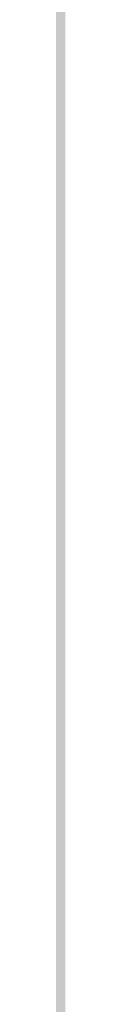
# Model space of a CAD drawing. Units: inches. Extents: x 2083 to 3317, y 1141 to 2115.
# Tile 219 of 256: x 3126.956 to 3126.958, y 1265.165 to 1267.234. Entities that reach past the tile are written whole.
import ezdxf

# ---------------------------------------------------------------- set-up
doc = ezdxf.new("R2010")
doc.units = ezdxf.units.IN
doc.layers.add('A-ANNO-DIMS', color=2, linetype='Continuous', lineweight=18)
doc.layers.add('A-WALL-PATT', color=251, linetype='Continuous', lineweight=13, true_color=0x636466)
doc.styles.get("Standard").update_dxf_attribs({"font": 'arial.ttf'})
doc.dimstyles.new('ISO-25', dxfattribs={"dimtxt": 12, "dimasz": 12, "dimexe": 1.25, "dimexo": 0.625, "dimtad": 1, "dimlunit": 3, "dimtxsty": 'Standard', "dimcen": 2.5, "dimadec": 0, "dimazin": 0, "dimtfac": 1, "dimtmove": 0, "dimatfit": 3, "dimfxl": 1, "dimarcsym": 0})

# ---------------------------------------------------------------- blocks, each defined once
blk = doc.blocks.new('*D26')
at = {"layer": 'A-ANNO-DIMS', "color": 0, "lineweight": -2, "transparency": 16777216}
for p, q in [((3088.9858, 1274.9151), (3088.9858, 1270.952)), ((3111.24, 1274.9151), (3111.24, 1270.952)), ((3076.9858, 1272.202), (2840.2624, 1272.202)), ((3111.24, 1272.202), (3088.9858, 1272.202)), ((3123.24, 1272.202), (3135.24, 1272.202))]:
    blk.add_line(p, q, dxfattribs=at)
at = {"layer": 'A-ANNO-DIMS', "color": 0, "transparency": 16777216}
for points in [[(3076.9858, 1274.202), (3076.9858, 1270.202), (3088.9858, 1272.202)], [(3123.24, 1274.202), (3123.24, 1270.202), (3111.24, 1272.202)]]:
    blk.add_solid(points, dxfattribs=at)
at = {"layer": 'Defpoints', "color": 0, "transparency": 16777216}
for p in [(3088.9858, 1275.5401), (3111.24, 1275.5401), (3088.9858, 1272.202)]:
    blk.add_point(p, dxfattribs=at)
at = {"layer": 'A-ANNO-DIMS', "color": 0, "transparency": 16777216, "insert": (2952.6241, 1279.0316), "char_height": 12, "attachment_point": 5}
blk.add_mtext('NIGHTSTAND 1\'-10 1/2" TYP.', dxfattribs=at)
blk = doc.blocks.new('*D27')
at = {"layer": 'A-ANNO-DIMS', "color": 0, "lineweight": -2, "transparency": 16777216}
for p, q in [((3114.5782, 1309.7943), (3114.5782, 1321.7943)), ((3111.865, 1297.7943), (3115.8282, 1297.7943)), ((3114.5782, 1297.7943), (3114.5782, 1275.5401)), ((3111.865, 1275.5401), (3115.8282, 1275.5401)), ((3114.5782, 1263.5401), (3114.5782, 1140.9886))]:
    blk.add_line(p, q, dxfattribs=at)
at = {"layer": 'A-ANNO-DIMS', "color": 0, "transparency": 16777216}
for points in [[(3112.5782, 1309.7943), (3116.5782, 1309.7943), (3114.5782, 1297.7943)], [(3112.5782, 1263.5401), (3116.5782, 1263.5401), (3114.5782, 1275.5401)]]:
    blk.add_solid(points, dxfattribs=at)
at = {"layer": 'Defpoints', "color": 0, "transparency": 16777216}
for p in [(3111.24, 1297.7943), (3111.24, 1275.5401), (3114.5782, 1275.5401)]:
    blk.add_point(p, dxfattribs=at)
at = {"layer": 'A-ANNO-DIMS', "color": 0, "transparency": 16777216, "insert": (3107.7485, 1196.2643), "char_height": 12, "attachment_point": 5, "rotation": 90}
blk.add_mtext('1\'-10 1/2" TYP.', dxfattribs=at)

msp = doc.modelspace()

# ---------------------------------------------------------------- hatches: boundary and pattern name
at = {"layer": 'A-WALL-PATT'}
h = msp.add_hatch(color=256, dxfattribs=at)
h.dxf.hatch_style = 1
h.paths.add_polyline_path([(3126.9598, 2020.7614), (2748.9598, 2020.7614), (2604.9598, 2020.7614), (2226.9598, 2020.7614), (2226.9598, 1702.7614), (2466.9598, 1702.7614), (2466.9598, 1582.7614), (2418.9598, 1582.7614), (2418.9598, 1477.7614), (2226.9598, 1477.7614), (2226.9598, 1263.2614), (2544.9598, 1263.2614), (2544.9598, 1411.7614), (2604.9598, 1411.7614), (2685.9598, 1411.7614), (2685.9598, 1420.7614), (2604.9598, 1420.7614), (2604.9598, 1573.7614), (2604.9598, 1702.7614), (2604.9598, 2011.7614), (2748.9598, 2011.7614), (2748.9598, 1702.7614), (2862.9598, 1702.7614), (2862.9598, 1621.7614), (2871.9598, 1621.7614), (2871.9598, 1702.7614), (2883.9598, 1702.7614), (2883.9598, 1706.9395, -0.026459), (2883.9598, 1711.7614), (2757.9598, 1711.7614), (2757.9598, 1807.7614), (2787.9598, 1807.7614), (2787.9598, 1812.2614), (2757.9598, 1812.2614), (2757.9598, 2011.7614), (2877.9598, 2011.7614), (2877.9598, 1812.2614), (2847.9598, 1812.2614), (2847.9598, 1807.7614), (2889.8357, 1807.7614), (2889.8357, 1812.2614), (2882.4598, 1812.2614), (2882.4598, 2011.7614), (3117.9598, 2011.7614), (3117.9598, 1812.2614), (2937.8357, 1812.2614), (2937.8357, 1807.7614), (2995.7098, 1807.7614), (2995.7098, 1796.1177), (3000.2098, 1796.1177), (3000.2098, 1807.7614), (3117.9598, 1807.7614), (3117.9598, 1711.7614), (3000.2098, 1711.7614), (3000.2098, 1760.1177), (2998.5727, 1760.1177, -0.020711), (2995.7098, 1760.1177), (2995.7098, 1711.7614), (2931.9598, 1711.7614), (2931.9598, 1702.7614), (3126.9598, 1702.7614)])
h.paths.add_polyline_path([(2471.4598, 2011.7614), (2471.4598, 1810.0114), (2462.7169, 1810.0114), (2462.7169, 1805.5114), (2505.9598, 1805.5114), (2505.9598, 1810.0114), (2475.9598, 1810.0114), (2475.9598, 2011.7614), (2595.9598, 2011.7614), (2595.9598, 1810.0114), (2565.9598, 1810.0114), (2565.9598, 1805.5114), (2595.9598, 1805.5114), (2595.9598, 1711.7614), (2235.9598, 1711.7614), (2235.9598, 1805.5114), (2353.7098, 1805.5114), (2353.7098, 1796.0542), (2358.2098, 1796.0542), (2358.2098, 1805.5114), (2414.7169, 1805.5114), (2414.7169, 1810.0114), (2235.9598, 1810.0114), (2235.9598, 2011.7614)], flags=16)
h.paths.add_polyline_path([(2270.2047, 1994.61), (2270.2047, 1970.61), (2246.2047, 1970.61), (2246.2047, 1994.61)], flags=0)
edge = h.paths.add_edge_path(flags=0)
edge.add_ellipse((2332.0274, 1899.7982), major_axis=(-3.043, 3.043), ratio=0.168252, start_angle=-161.3322, end_angle=-156.3071, ccw=False)
edge.add_ellipse((2333.082, 1898.7435), major_axis=(-1.0546, 1.0546), ratio=0.453532, start_angle=-123.371, end_angle=-94.1591)
edge = h.paths.add_edge_path(flags=0)
edge.add_ellipse((2332.0274, 1968.8763), major_axis=(3.043, 3.043), ratio=0.168252, start_angle=18.6678, end_angle=23.6929)
edge.add_spline(control_points=[(2332.9256, 1970.6911), (2332.2268, 1970.3361), (2330.8937, 1969.6589), (2328.4131, 1970.9321), (2327.2039, 1967.7487), (2324.7096, 1969.9556), (2322.5328, 1967.0124), (2320.0128, 1971.2958), (2317.6803, 1968.1578), (2316.0405, 1967.102), (2315.4269, 1966.8096)], knot_values=[0, 0, 0, 0, 2.267059, 4.324559, 6.685584, 8.878641, 11.121502, 14.300359, 17.755284, 19.732645, 19.732645, 19.732645, 19.732645], degree=3, periodic=0)
edge.add_ellipse((2332.0274, 1968.8763), major_axis=(3.043, 3.043), ratio=0.168252, start_angle=18.6678, end_angle=23.6929, ccw=False)
edge.add_ellipse((2333.082, 1969.9309), major_axis=(1.0546, 1.0546), ratio=0.453532, start_angle=56.629, end_angle=85.8409, ccw=False)
edge = h.paths.add_edge_path(flags=0)
edge.add_spline(control_points=[(2296.4283, 1967.9879), (2293.6278, 1965.3363), (2287.7036, 1959.7271), (2299.7439, 1949.9957), (2294.5326, 1935.6685), (2290.5732, 1920.6035), (2293.3941, 1909.9737), (2296.1854, 1904.9665)], knot_values=[0.099185, 0.099185, 0.099185, 0.099185, 0.345301, 0.619822, 0.982653, 1.386093, 1.810555, 1.810555, 1.810555, 1.810555], degree=3, periodic=0)
edge.add_spline(control_points=[(2296.1854, 1904.9665), (2297.3836, 1902.6193), (2298.001, 1901.9493), (2298.553, 1901.4682)], knot_values=[0.006246, 0.006246, 0.006246, 0.006246, 0.055476, 0.055476, 0.055476, 0.055476], degree=3, periodic=0)
edge.add_spline(control_points=[(2298.553, 1901.4682), (2297.2586, 1900.9232), (2295.2253, 1900.2321), (2293.0602, 1900.6142), (2292.1014, 1900.7884), (2292.0896, 1900.7906)], knot_values=[0.312835, 0.312835, 0.312835, 0.312835, 0.40178, 0.474987, 0.475903, 0.475903, 0.475903, 0.475903], degree=3, periodic=0)
edge.add_arc((2292.7936, 1904.6641), 3.937, 215.4209, 259.6982, ccw=False)
edge.add_spline(control_points=[(2289.5853, 1902.3823), (2289.4767, 1902.5351), (2289.3685, 1902.688), (2289.2609, 1902.8412)], knot_values=[0.102872, 0.102872, 0.102872, 0.102872, 0.116896, 0.116896, 0.116896, 0.116896], degree=3, periodic=0)
edge.add_spline(control_points=[(2289.2609, 1902.8412), (2288.6866, 1902.5502), (2287.64, 1902.0199), (2285.8813, 1901.874), (2283.853, 1901.5044), (2281.72, 1899.7105), (2278.467, 1899.4929), (2276.1571, 1901.8832), (2272.259, 1899.8041), (2267.7776, 1901.8432), (2262.2439, 1900.184), (2257.4149, 1901.7821), (2254.3184, 1900.7261), (2253.1783, 1900.3373)], knot_values=[0, 0, 0, 0, 1.907977, 3.477176, 5.261074, 7.972851, 11.680248, 13.717921, 16.939592, 22.789562, 27.502503, 33.595215, 37.145618, 37.145618, 37.145618, 37.145618], degree=3, periodic=0)
edge.add_line((2253.1783, 1900.3373), (2250.2442, 1902.8412))
edge.add_line((2250.2442, 1902.8412), (2250.2442, 1965.8333))
edge.add_line((2250.2442, 1965.8333), (2253.1783, 1968.3371))
edge.add_spline(control_points=[(2253.1783, 1968.3371), (2254.3184, 1967.9483), (2257.4149, 1966.8924), (2262.2439, 1968.4904), (2267.7776, 1966.8313), (2271.5267, 1968.5372), (2273.8759, 1967.8283), (2274.2067, 1967.7276)], knot_values=[0, 0, 0, 0, 0.09018, 0.244935, 0.364644, 0.513233, 0.537855, 0.537855, 0.537855, 0.537855], degree=3, periodic=0)
edge.add_arc((2274.3529, 1963.7933), 3.937, 72.0511, 92.1279, ccw=False)
edge.add_arc((2281.2969, 1985.23), 18.5963, 252.05113, 288.56572)
edge.add_arc((2292.3167, 1956.0289), 12.6461, 71.02679, 113.77822, ccw=False)
edge = h.paths.add_edge_path(flags=0)
edge.add_spline(control_points=[(2274.8994, 1951.8562), (2275.0662, 1951.6166), (2275.2327, 1951.3766), (2275.398, 1951.1359)], knot_values=[1.409916, 1.409916, 1.409916, 1.409916, 1.43159, 1.43159, 1.43159, 1.43159], degree=3, periodic=0)
edge.add_spline(control_points=[(2275.398, 1951.1359), (2275.7921, 1950.5619), (2276.1792, 1949.9838), (2276.5455, 1949.3971)], knot_values=[1.358238, 1.358238, 1.358238, 1.358238, 1.409916, 1.409916, 1.409916, 1.409916], degree=3, periodic=0)
edge.add_line((2276.5455, 1949.3971), (2277.4373, 1947.8622))
edge.add_spline(control_points=[(2277.4373, 1947.8622), (2276.3038, 1945.6731), (2274.6397, 1942.4269), (2274.6316, 1938.0939), (2272.7991, 1930.8515), (2274.3564, 1943.897), (2275.9477, 1947.9234), (2276.5455, 1949.3971)], knot_values=[0.005632, 0.005632, 0.005632, 0.005632, 0.186014, 0.266002, 0.357087, 0.59639, 0.739732, 0.739732, 0.739732, 0.739732], degree=3, periodic=0)
edge.add_spline(control_points=[(2276.5455, 1949.3971), (2276.1792, 1949.9838), (2275.7921, 1950.5619), (2275.398, 1951.1359)], knot_values=[1.358238, 1.358238, 1.358238, 1.358238, 1.409916, 1.409916, 1.409916, 1.409916], degree=3, periodic=0)
edge.add_spline(control_points=[(2275.398, 1951.1359), (2274.9425, 1950.0805), (2274.2078, 1948.0253), (2273.9346, 1944.8515), (2272.4685, 1937.6275), (2273.4662, 1945.6965), (2274.7006, 1951.0595), (2274.8994, 1951.8562)], knot_values=[0.104364, 0.104364, 0.104364, 0.104364, 0.189636, 0.269624, 0.36071, 0.600013, 0.644622, 0.644622, 0.644622, 0.644622], degree=3, periodic=0)
h.paths.add_polyline_path([(2269.1675, 1963.1276, -0.357527), (2268.1706, 1960.9764, -0.092561), (2268.1706, 1939.4363, -0.357527), (2269.1675, 1937.2851, -0.357527), (2267.0163, 1938.282, -0.164785), (2254.6856, 1938.282, -0.357527), (2252.5344, 1937.2851, -0.357527), (2253.5313, 1939.4363, -0.092561), (2253.5313, 1960.9764, -0.357527), (2252.5344, 1963.1276, -0.357527), (2254.6856, 1962.1307, -0.164785), (2267.0163, 1962.1307, -0.357527)], flags=0)
h.paths.add_polyline_path([(2248.8741, 1967.8018), (2248.8741, 1957.0277), (2249.4578, 1957.0277), (2249.4578, 1911.6468), (2248.8741, 1911.6468), (2248.8741, 1900.8727), (2246.5119, 1900.8727, 0.197327), (2244.1497, 1902.4569), (2244.1497, 1966.2176, 0.197327), (2246.5119, 1967.8018)], flags=0)
h.paths.add_polyline_path([(2269.1675, 1931.3893, -0.357527), (2268.1706, 1929.2381, -0.092561), (2268.1706, 1907.6981, -0.357527), (2269.1675, 1905.5469, -0.357527), (2267.0163, 1906.5438, -0.164785), (2254.6856, 1906.5438, -0.357527), (2252.5344, 1905.5469, -0.357527), (2253.5313, 1907.6981, -0.092561), (2253.5313, 1929.2381, -0.357527), (2252.5344, 1931.3893, -0.357527), (2254.6856, 1930.3925, -0.164785), (2267.0163, 1930.3925, -0.357527)], flags=0)
edge = h.paths.add_edge_path(flags=0)
edge.add_spline(control_points=[(2276.1969, 1906.7237), (2276.1681, 1909.0289), (2276.114, 1913.3719), (2270.5984, 1924.925), (2273.9052, 1919.0128), (2275.9217, 1916.2621), (2275.4746, 1912.4021), (2277.2579, 1910.3806), (2276.696, 1908.225), (2276.6462, 1906.813), (2276.6178, 1906.0084)], knot_values=[0, 0, 0, 0, 8.61026, 16.221274, 18.843057, 23.804898, 27.440828, 29.356102, 31.203478, 33.650687, 33.650687, 33.650687, 33.650687], degree=3, periodic=0)
edge.add_spline(control_points=[(2276.6178, 1906.0084), (2276.6233, 1905.6241), (2276.4977, 1904.6287), (2275.4418, 1903.8547), (2274.9373, 1903.0804), (2274.8591, 1902.8412)], knot_values=[0.156488, 0.156488, 0.156488, 0.156488, 0.184398, 0.231376, 0.250598, 0.250598, 0.250598, 0.250598], degree=3, periodic=0)
edge.add_line((2274.8591, 1902.8412), (2276.506, 1902.8412))
edge.add_spline(control_points=[(2276.506, 1902.8412), (2276.7883, 1903.0849), (2277.6651, 1904.1252), (2278.2495, 1904.3407), (2277.6539, 1908.5274), (2278.1557, 1906.2278), (2278.1005, 1905.2859), (2278.8467, 1904.069), (2277.8568, 1903.4149), (2277.8742, 1902.991), (2277.9036, 1902.8412)], knot_values=[0.059574, 0.059574, 0.059574, 0.059574, 0.080753, 0.103741, 0.16972, 0.176036, 0.207137, 0.240474, 0.262341, 0.27366, 0.27366, 0.27366, 0.27366], degree=3, periodic=0)
edge.add_line((2277.9036, 1902.8412), (2280.0298, 1902.8412))
edge.add_spline(control_points=[(2280.0298, 1902.8412), (2279.8882, 1903.0884), (2279.4993, 1903.9816), (2280.1523, 1905.9393), (2278.1036, 1909.6578), (2279.7624, 1907.1853), (2280.3279, 1904.8749), (2280.4851, 1903.4896), (2281.4633, 1903.2494), (2281.7583, 1902.9365), (2281.834, 1902.8412)], knot_values=[0.013856, 0.013856, 0.013856, 0.013856, 0.034874, 0.088867, 0.107879, 0.126738, 0.158714, 0.193757, 0.217487, 0.226722, 0.226722, 0.226722, 0.226722], degree=3, periodic=0)
edge.add_spline(control_points=[(2281.834, 1902.8412), (2281.7875, 1902.8267), (2281.647, 1902.783), (2281.3955, 1902.8595), (2281.0881, 1902.9852), (2280.7207, 1903.0609), (2280.3335, 1903.0257), (2280.1248, 1902.8989), (2280.0298, 1902.8412)], knot_values=[0, 0, 0, 0, 0.14413, 0.435517, 0.749276, 1.153046, 1.548371, 1.878348, 1.878348, 1.878348, 1.878348], degree=3, periodic=0)
edge.add_line((2280.0298, 1902.8412), (2277.9036, 1902.8412))
edge.add_spline(control_points=[(2277.9036, 1902.8412), (2277.8929, 1902.7959), (2277.8654, 1902.6796), (2277.6075, 1902.6875), (2277.2741, 1902.8007), (2276.8379, 1902.6198), (2276.5838, 1902.7893), (2276.506, 1902.8412)], knot_values=[0, 0, 0, 0, 0.127189, 0.326199, 0.628009, 1.24357, 1.515331, 1.515331, 1.515331, 1.515331], degree=3, periodic=0)
edge.add_line((2276.506, 1902.8412), (2274.8591, 1902.8412))
edge.add_spline(control_points=[(2274.8591, 1902.8412), (2274.8144, 1902.8986), (2274.7251, 1903.0134), (2274.4935, 1903.119), (2274.2443, 1902.9605), (2273.9371, 1903.1849), (2273.614, 1902.9831), (2273.4083, 1902.883), (2273.3223, 1902.8412)], knot_values=[0, 0, 0, 0, 0.21843, 0.436957, 0.687977, 0.990379, 1.398396, 1.69185, 1.69185, 1.69185, 1.69185], degree=3, periodic=0)
edge.add_spline(control_points=[(2273.3223, 1902.8412), (2273.6167, 1903.4457), (2274.274, 1904.5383), (2276.0272, 1904.5737), (2276.207, 1906.5836), (2276.1969, 1906.7237)], knot_values=[0.012227, 0.012227, 0.012227, 0.012227, 0.059472, 0.106218, 0.134458, 0.134458, 0.134458, 0.134458], degree=3, periodic=0)
h.paths.add_polyline_path([(2270.7761, 1897.7898), (2270.7761, 1873.7898), (2246.7761, 1873.7898), (2246.7761, 1897.7898)], flags=0)
h.paths.add_polyline_path([(2353.7098, 1760.0051), (2353.7098, 1760.0542), (2358.2098, 1760.0542, -0.033729)], flags=0)
h.paths.add_polyline_path([(2321.8191, 1737.5292), (2341.9953, 1737.5292, -0.414214), (2343.2033, 1736.3212), (2343.2033, 1721.0206, -0.414214), (2341.9953, 1719.8127), (2321.8191, 1719.8127, -0.414214), (2320.6112, 1721.0206), (2320.6112, 1736.3212, -0.414214)], flags=0)
h.paths.add_polyline_path([(2324.235, 1736.3212), (2339.5794, 1736.3212, -0.414214), (2341.9953, 1733.9053), (2341.9953, 1725.4497, -0.414214), (2339.5794, 1723.0338), (2333.6806, 1723.0338), (2333.8453, 1722.0455, -0.870646), (2335.4254, 1721.8259, -0.767327), (2333.9227, 1721.4232), (2331.291, 1721.4232, -0.767327), (2329.7883, 1721.8259, -0.870646), (2331.3684, 1722.0455), (2331.5331, 1723.0338), (2324.235, 1723.0338, -0.414214), (2321.8191, 1725.4497), (2321.8191, 1733.9053, -0.414214)], flags=0)
h.paths.add_polyline_path([(2570.4838, 1928.6154), (2589.6838, 1928.6154), (2590.1688, 1928.6154), (2590.1688, 1904.9934), (2570.4838, 1904.9934)], flags=0)
h.paths.add_polyline_path([(2574.4473, 1927.2638, -1), (2572.8288, 1927.2638, -1)], flags=0)
h.paths.add_polyline_path([(2573.0899, 1926.9409), (2573.925, 1927.776), (2574.1477, 1927.5533), (2573.3126, 1926.7182)], flags=0)
h.paths.add_polyline_path([(2578.7791, 1919.7296, -1), (2571.5917, 1919.7296, -1)], flags=0)
h.paths.add_polyline_path([(2578.3854, 1919.7296, -1), (2571.9854, 1919.7296, -1)], flags=0)
h.paths.add_polyline_path([(2331.5958, 1729.4762, -1), (2333.618, 1729.4762, -1)], flags=0)
h.paths.add_polyline_path([(2578.0342, 1927.2638, -1), (2576.4157, 1927.2638, -1)], flags=0)
h.paths.add_polyline_path([(2576.6889, 1927.5311), (2576.9116, 1927.7538), (2577.7467, 1926.9186), (2577.524, 1926.6959)], flags=0)
h.paths.add_polyline_path([(2578.1391, 1909.8595, -1), (2572.2317, 1909.8595, -1)], flags=0)
h.paths.add_polyline_path([(2577.7454, 1909.8595, -1), (2572.6254, 1909.8595, -1)], flags=0)
h.paths.add_polyline_path([(2583.7977, 1927.2638, -1), (2582.1792, 1927.2638, -1)], flags=0)
h.paths.add_polyline_path([(2582.7186, 1927.7538), (2583.5538, 1926.9186), (2583.3311, 1926.6959), (2582.4959, 1927.5311)], flags=0)
h.paths.add_polyline_path([(2582.4959, 1927.5311), (2582.7186, 1927.7538), (2583.5538, 1926.9186), (2583.3311, 1926.6959)], flags=0)
h.paths.add_polyline_path([(2587.7391, 1920.5296, -1), (2581.8317, 1920.5296, -1)], flags=0)
h.paths.add_polyline_path([(2587.3454, 1920.5296, -1), (2582.2254, 1920.5296, -1)], flags=0)
h.paths.add_polyline_path([(2587.3846, 1927.2638, -1), (2585.7661, 1927.2638, -1)], flags=0)
h.paths.add_polyline_path([(2586.082, 1926.9802), (2586.9172, 1927.8154), (2587.1399, 1927.5927), (2586.3047, 1926.7575)], flags=0)
h.paths.add_polyline_path([(2588.3791, 1910.6595, -1), (2581.1917, 1910.6595, -1)], flags=0)
h.paths.add_polyline_path([(2587.9854, 1910.6595, -1), (2581.5854, 1910.6595, -1)], flags=0)
h.paths.add_polyline_path([(2417.1677, 1729.4779), (2437.3439, 1729.4779, -0.414214), (2438.5519, 1728.2699), (2438.5519, 1712.9693, -0.414214), (2437.3439, 1711.7614), (2417.1677, 1711.7614, -0.414214), (2415.9598, 1712.9693), (2415.9598, 1728.2699, -0.414214)], flags=0)
h.paths.add_polyline_path([(2419.5836, 1728.2699), (2434.928, 1728.2699, -0.414214), (2437.3439, 1725.8541), (2437.3439, 1717.3984, -0.414214), (2434.928, 1714.9825), (2429.0292, 1714.9825), (2429.1939, 1713.9942, -0.870646), (2430.774, 1713.7746, -0.767327), (2429.2713, 1713.372), (2426.6396, 1713.372, -0.767327), (2425.1369, 1713.7746, -0.870646), (2426.717, 1713.9942), (2426.8817, 1714.9825), (2419.5836, 1714.9825, -0.414214), (2417.1677, 1717.3984), (2417.1677, 1725.8541, -0.414214)], flags=0)
h.paths.add_polyline_path([(2419.5836, 1728.2699), (2434.928, 1728.2699, -0.414214), (2437.3439, 1725.8541), (2437.3439, 1717.3984, -0.414214), (2434.928, 1714.9825), (2429.0292, 1714.9825), (2428.3581, 1719.009), (2427.5528, 1719.009), (2426.8817, 1714.9825), (2419.5836, 1714.9825, -0.414214), (2417.1677, 1717.3984), (2417.1677, 1725.8541, -0.414214)], flags=0)
h.paths.add_polyline_path([(2426.9444, 1721.4249, -1), (2428.9666, 1721.4249, -1)], flags=0)
h.paths.add_polyline_path([(2475.9598, 1702.7614), (2595.9598, 1702.7614), (2595.9598, 1582.7614), (2475.9598, 1582.7614)], flags=16)
h.paths.add_polyline_path([(2427.9598, 1573.7614), (2595.9598, 1573.7614), (2595.9598, 1468.7614), (2595.9598, 1420.7614), (2384.4598, 1420.7614), (2384.4598, 1468.7614), (2427.9598, 1468.7614)], flags=16)
h.paths.add_polyline_path([(2379.9598, 1468.7614), (2379.9598, 1420.7614), (2235.9598, 1420.7614), (2235.9598, 1468.7614)], flags=16)
h.paths.add_polyline_path([(2317.816, 1466.6958), (2337.9922, 1466.6958, -0.414214), (2339.2002, 1465.4878), (2339.2002, 1450.1872, -0.414214), (2337.9922, 1448.9792), (2317.816, 1448.9792, -0.414214), (2316.6081, 1450.1872), (2316.6081, 1465.4878, -0.414214)], flags=0)
h.paths.add_polyline_path([(2320.2319, 1465.4878), (2335.5763, 1465.4878, -0.414214), (2337.9922, 1463.0719), (2337.9922, 1454.6163, -0.414214), (2335.5763, 1452.2004), (2329.6775, 1452.2004), (2329.8422, 1451.212, -0.870646), (2331.4223, 1450.9925, -0.767327), (2329.9196, 1450.5898), (2327.2879, 1450.5898, -0.767327), (2325.7852, 1450.9925, -0.870646), (2327.3653, 1451.212), (2327.53, 1452.2004), (2320.2319, 1452.2004, -0.414214), (2317.816, 1454.6163), (2317.816, 1463.0719, -0.414214)], flags=0)
h.paths.add_polyline_path([(2320.2319, 1465.4878), (2335.5763, 1465.4878, -0.414214), (2337.9922, 1463.0719), (2337.9922, 1454.6163, -0.414214), (2335.5763, 1452.2004), (2329.6775, 1452.2004), (2329.0064, 1456.2269), (2328.2011, 1456.2269), (2327.53, 1452.2004), (2320.2319, 1452.2004, -0.414214), (2317.816, 1454.6163), (2317.816, 1463.0719, -0.414214)], flags=0)
h.paths.add_polyline_path([(2327.5926, 1458.6428, -1), (2329.6148, 1458.6428, -1)], flags=0)
h.paths.add_polyline_path([(2244.4117, 1433.3405), (2241.9209, 1433.3405, -0.414214), (2240.0179, 1435.2435), (2240.0179, 1440.9528, -0.414211), (2241.9209, 1442.8559), (2244.4117, 1442.8559, -1.976472)], flags=0)
h.paths.add_polyline_path([(2245.3569, 1434.3975, -0.414214), (2245.3569, 1441.7988, -2.144098)], flags=0)
h.paths.add_polyline_path([(2535.9598, 1416.2614), (2535.9598, 1272.2614), (2235.9598, 1272.2614), (2235.9598, 1416.2614)], flags=16)
h.paths.add_polyline_path([(2260.1196, 1384.2928), (2260.1196, 1362.0386), (2237.8654, 1362.0386), (2237.8654, 1384.2928)], flags=0)
edge = h.paths.add_edge_path(flags=0)
edge.add_line((2318.2518, 1362.0933), (2318.1458, 1362.001))
edge.add_ellipse((2317.4451, 1360.431), major_axis=(2.8216, 2.8216), ratio=0.168252, start_angle=18.6678, end_angle=20.9481, ccw=False)
edge.add_ellipse((2318.423, 1361.409), major_axis=(0.9779, 0.9779), ratio=0.453532, start_angle=56.629, end_angle=70.2262, ccw=False)
edge = h.paths.add_edge_path(flags=0)
edge.add_line((2319.1074, 1295.5711), (2319.015, 1295.6771))
edge.add_ellipse((2317.4451, 1296.3778), major_axis=(-2.8216, 2.8216), ratio=0.168252, start_angle=-161.3322, end_angle=-159.0519, ccw=False)
edge.add_ellipse((2318.423, 1295.3999), major_axis=(-0.9779, 0.9779), ratio=0.453532, start_angle=-123.371, end_angle=-109.7738)
edge = h.paths.add_edge_path(flags=0)
edge.add_spline(control_points=[(2284.2103, 1301.1702), (2284.5807, 1300.4447), (2284.8912, 1299.892), (2285.1596, 1299.461)], knot_values=[0.039066, 0.039066, 0.039066, 0.039066, 0.055476, 0.055476, 0.055476, 0.055476], degree=3, periodic=0)
edge.add_line((2285.1596, 1299.461), (2284.2103, 1301.1702))
edge = h.paths.add_edge_path(flags=0)
edge.add_line((2280.4125, 1297.298), (2283.37, 1297.0361))
edge.add_line((2283.37, 1297.0361), (2286.4057, 1297.9263))
edge.add_spline(control_points=[(2286.4057, 1297.9263), (2285.3055, 1297.4631), (2284.3448, 1297.1292), (2283.37, 1297.0361)], knot_values=[0.394369, 0.394369, 0.394369, 0.394369, 0.475903, 0.475903, 0.475903, 0.475903], degree=3, periodic=0)
edge.add_spline(control_points=[(2283.37, 1297.0361), (2283.2814, 1297.0277), (2282.3163, 1296.9573), (2281.3125, 1297.1345), (2280.4234, 1297.296), (2280.4125, 1297.298)], knot_values=[0.312835, 0.312835, 0.312835, 0.312835, 0.320246, 0.393453, 0.394369, 0.394369, 0.394369, 0.394369], degree=3, periodic=0)
edge = h.paths.add_edge_path(flags=0)
edge.add_line((2284.4356, 1359.6073), (2280.4463, 1355.328))
edge.add_line((2280.4463, 1355.328), (2279.58, 1351.0178))
edge.add_line((2279.58, 1351.0178), (2282.413, 1346.5804))
edge.add_spline(control_points=[(2282.413, 1346.5804), (2283.1533, 1345.5892), (2284.2529, 1344.0289), (2284.801, 1342.3872), (2284.9352, 1341.8055)], knot_values=[1.240098, 1.240098, 1.240098, 1.240098, 1.332892, 1.382712, 1.382712, 1.382712, 1.382712], degree=3, periodic=0)
edge.add_spline(control_points=[(2284.9352, 1341.8055), (2285.3191, 1340.1406), (2285.233, 1338.4092), (2284.9099, 1336.6541)], knot_values=[1.097484, 1.097484, 1.097484, 1.097484, 1.240098, 1.240098, 1.240098, 1.240098], degree=3, periodic=0)
edge.add_spline(control_points=[(2284.9099, 1336.6541), (2284.5868, 1334.899), (2284.0267, 1333.1203), (2283.4626, 1331.3606)], knot_values=[0.95487, 0.95487, 0.95487, 0.95487, 1.097484, 1.097484, 1.097484, 1.097484], degree=3, periodic=0)
edge.add_line((2283.4626, 1331.3606), (2281.8904, 1326.1534))
edge.add_line((2281.8904, 1326.1534), (2280.7563, 1321.0561))
edge.add_line((2280.7563, 1321.0561), (2280.2992, 1316.002))
edge.add_line((2280.2992, 1316.002), (2280.7159, 1310.9501))
edge.add_line((2280.7159, 1310.9501), (2282.0281, 1305.9721))
edge.add_line((2282.0281, 1305.9721), (2284.2103, 1301.1702))
edge.add_spline(control_points=[(2284.2103, 1301.1702), (2283.3407, 1302.7302), (2282.6119, 1304.3365), (2282.0281, 1305.9721)], knot_values=[0.099185, 0.099185, 0.099185, 0.099185, 0.241799, 0.241799, 0.241799, 0.241799], degree=3, periodic=0)
edge.add_spline(control_points=[(2282.0281, 1305.9721), (2281.4443, 1307.6078), (2281.0055, 1309.2728), (2280.7159, 1310.9501)], knot_values=[0.241799, 0.241799, 0.241799, 0.241799, 0.384413, 0.384413, 0.384413, 0.384413], degree=3, periodic=0)
edge.add_spline(control_points=[(2280.7159, 1310.9501), (2280.4332, 1312.5876), (2280.2894, 1314.277), (2280.2989, 1315.962), (2280.2992, 1316.002)], knot_values=[0.384413, 0.384413, 0.384413, 0.384413, 0.523647, 0.527028, 0.527028, 0.527028, 0.527028], degree=3, periodic=0)
edge.add_spline(control_points=[(2280.2992, 1316.002), (2280.3123, 1317.687), (2280.4779, 1319.3679), (2280.7563, 1321.0561)], knot_values=[0.527028, 0.527028, 0.527028, 0.527028, 0.669642, 0.669642, 0.669642, 0.669642], degree=3, periodic=0)
edge.add_spline(control_points=[(2280.7563, 1321.0561), (2281.0346, 1322.7443), (2281.4259, 1324.4396), (2281.8904, 1326.1534)], knot_values=[0.669642, 0.669642, 0.669642, 0.669642, 0.812256, 0.812256, 0.812256, 0.812256], degree=3, periodic=0)
edge.add_spline(control_points=[(2281.8904, 1326.1534), (2282.2644, 1327.5333), (2282.7879, 1329.2618), (2283.3528, 1331.0178), (2283.4626, 1331.3606)], knot_values=[0.812256, 0.812256, 0.812256, 0.812256, 0.927087, 0.95487, 0.95487, 0.95487, 0.95487], degree=3, periodic=0)
edge.add_line((2283.4626, 1331.3606), (2284.9099, 1336.6541))
edge.add_line((2284.9099, 1336.6541), (2284.9352, 1341.8055))
edge.add_line((2284.9352, 1341.8055), (2282.413, 1346.5804))
edge.add_spline(control_points=[(2282.413, 1346.5804), (2281.2751, 1348.1038), (2280.0784, 1349.5703), (2279.58, 1351.0178)], knot_values=[1.382712, 1.382712, 1.382712, 1.382712, 1.525326, 1.525326, 1.525326, 1.525326], degree=3, periodic=0)
edge.add_spline(control_points=[(2279.58, 1351.0178), (2279.4433, 1351.4147), (2279.1363, 1352.8569), (2279.7352, 1354.2904), (2280.4463, 1355.328)], knot_values=[1.525326, 1.525326, 1.525326, 1.525326, 1.564439, 1.667941, 1.667941, 1.667941, 1.667941], degree=3, periodic=0)
edge.add_spline(control_points=[(2280.4463, 1355.328), (2281.4261, 1356.7578), (2282.9308, 1358.1826), (2284.4356, 1359.6073)], knot_values=[1.667941, 1.667941, 1.667941, 1.667941, 1.810555, 1.810555, 1.810555, 1.810555], degree=3, periodic=0)
edge.add_arc((2280.6231, 1348.5182), 11.7262, 71.02679, 113.77822)
edge.add_arc((2270.4049, 1375.5952), 17.2436, 252.05113, 288.56572, ccw=False)
edge.add_arc((2263.966, 1355.7178), 3.6506, 72.0511, 92.1279)
edge.add_arc((2263.966, 1355.7178), 3.6506, 92.1279, 177.9851)
edge.add_spline(control_points=[(2260.3176, 1355.8462), (2260.2604, 1354.2207), (2260.5513, 1350.1865), (2262.9993, 1346.7663), (2264.4727, 1344.649)], knot_values=[1.43159, 1.43159, 1.43159, 1.43159, 1.564144, 1.770695, 1.770695, 1.770695, 1.770695], degree=3, periodic=0)
edge.add_line((2264.4727, 1344.649), (2264.9356, 1343.9825))
edge.add_spline(control_points=[(2263.801, 1340.2481), (2263.8432, 1340.5141), (2264.0672, 1341.7565), (2264.5127, 1343.0025), (2264.935, 1343.9811)], knot_values=[0.53657, 0.53657, 0.53657, 0.53657, 0.559349, 0.644622, 0.644622, 0.644622, 0.644622], degree=3, periodic=0)
edge.add_spline(control_points=[(2264.935, 1343.9811), (2265.1178, 1343.715), (2265.2989, 1343.4479), (2265.4768, 1343.1794)], knot_values=[1.384077, 1.384077, 1.384077, 1.384077, 1.409916, 1.409916, 1.409916, 1.409916], degree=3, periodic=0)
edge.add_spline(control_points=[(2265.4768, 1343.1794), (2265.6546, 1342.9108), (2265.8293, 1342.6408), (2265.9991, 1342.3688)], knot_values=[1.358238, 1.358238, 1.358238, 1.358238, 1.384077, 1.384077, 1.384077, 1.384077], degree=3, periodic=0)
edge.add_line((2265.9991, 1342.3688), (2266.826, 1340.9455))
edge.add_spline(control_points=[(2266.826, 1340.9455), (2268.8944, 1337.0897), (2271.3982, 1325.843), (2270.5162, 1310.5686), (2275.9194, 1301.8606), (2277.7895, 1299.1994)], knot_values=[0.116896, 0.116896, 0.116896, 0.116896, 0.472987, 1.050969, 1.313793, 1.313793, 1.313793, 1.313793], degree=3, periodic=0)
edge.add_spline(control_points=[(2277.7895, 1299.1994), (2277.8394, 1299.1285), (2277.8894, 1299.0575), (2277.9396, 1298.9866)], knot_values=[0.109884, 0.109884, 0.109884, 0.109884, 0.116896, 0.116896, 0.116896, 0.116896], degree=3, periodic=0)
edge.add_line((2277.9396, 1298.9866), (2277.7888, 1299.1991))
edge.add_spline(control_points=[(2277.7888, 1299.1991), (2277.2566, 1298.9294), (2276.2864, 1298.4379), (2275.0394, 1298.3344), (2274.3833, 1298.2389), (2274.2153, 1298.2093)], knot_values=[33.12187, 33.12187, 33.12187, 33.12187, 35.029056, 36.598255, 37.144827, 37.144827, 37.144827, 37.144827], degree=3, periodic=0)
edge.add_line((2274.2153, 1298.2093), (2273.0731, 1297.893))
edge.add_spline(control_points=[(2273.0731, 1297.893), (2272.3229, 1297.5798), (2271.0392, 1296.5105), (2269.2484, 1296.2261), (2268.4231, 1296.3747)], knot_values=[26.532584, 26.532584, 26.532584, 26.532584, 29.198919, 31.839101, 31.839101, 31.839101, 31.839101], degree=3, periodic=0)
edge.add_line((2268.4231, 1296.3747), (2263.8785, 1297.4575))
edge.add_spline(control_points=[(2263.8785, 1297.4575), (2263.5561, 1297.3594), (2261.8603, 1296.8387), (2260.2388, 1297.2824), (2258.9335, 1297.5165)], knot_values=[15.919551, 15.919551, 15.919551, 15.919551, 16.939592, 21.226067, 21.226067, 21.226067, 21.226067], degree=3, periodic=0)
edge.add_line((2258.9335, 1297.5165), (2254.0552, 1297.329))
edge.add_spline(control_points=[(2254.0552, 1297.329), (2253.7555, 1297.2958), (2252.1137, 1297.1652), (2250.4619, 1297.5442), (2249.1297, 1297.6679)], knot_values=[5.306517, 5.306517, 5.306517, 5.306517, 6.276435, 10.613034, 10.613034, 10.613034, 10.613034], degree=3, periodic=0)
edge.add_line((2249.1297, 1297.6679), (2244.3316, 1296.8778))
edge.add_line((2244.3316, 1296.8778), (2241.611, 1299.1994))
edge.add_line((2241.611, 1299.1994), (2241.611, 1357.6094))
edge.add_line((2241.611, 1357.6094), (2244.3316, 1359.9311))
edge.add_line((2244.3316, 1359.9311), (2252.7288, 1359.5427))
edge.add_spline(control_points=[(2252.7288, 1359.5427), (2252.8709, 1359.5464), (2253.3057, 1359.5482), (2253.7398, 1359.5143), (2254.0317, 1359.4824)], knot_values=[0.233291, 0.233291, 0.233291, 0.233291, 0.244935, 0.268927, 0.268927, 0.268927, 0.268927], degree=3, periodic=0)
edge.add_line((2254.0317, 1359.4824), (2259.5872, 1359.4164))
edge.add_spline(control_points=[(2259.5872, 1359.4164), (2260.6771, 1359.6285), (2262.0732, 1359.897), (2263.5237, 1359.4593), (2263.8304, 1359.366)], knot_values=[0.422516, 0.422516, 0.422516, 0.422516, 0.513233, 0.537855, 0.537855, 0.537855, 0.537855], degree=3, periodic=0)
edge.add_arc((2263.966, 1355.7178), 3.6506, 72.0511, 92.1279, ccw=False)
edge.add_arc((2270.4049, 1375.5952), 17.2436, 252.05113, 288.56572)
edge.add_arc((2280.6231, 1348.5182), 11.7262, 71.02679, 113.77822, ccw=False)
h.paths.add_polyline_path([(2240.3405, 1359.4347), (2240.3405, 1349.4444), (2240.8818, 1349.4444), (2240.8818, 1307.3645), (2240.3405, 1307.3645), (2240.3405, 1297.3741), (2238.1502, 1297.3741, 0.197327), (2235.9598, 1298.8431), (2235.9598, 1357.9657, 0.197327), (2238.1502, 1359.4347)], flags=0)
h.paths.add_polyline_path([(2259.1578, 1355.1005, -0.357527), (2258.2334, 1353.1058, -0.092561), (2258.2334, 1333.1326, -0.357527), (2259.1578, 1331.1379, -0.357527), (2257.1631, 1332.0622, -0.164785), (2245.7293, 1332.0622, -0.357527), (2243.7346, 1331.1379, -0.357527), (2244.6589, 1333.1326, -0.092561), (2244.6589, 1353.1058, -0.357527), (2243.7346, 1355.1005, -0.357527), (2245.7293, 1354.1761, -0.164785), (2257.1631, 1354.1761, -0.357527)], flags=0)
edge = h.paths.add_edge_path(flags=0)
edge.add_line((2265.9991, 1342.3688), (2266.826, 1340.9455))
edge.add_line((2266.826, 1340.9455), (2265.3076, 1337.8141))
edge.add_line((2265.3076, 1337.8141), (2264.3582, 1334.6529))
edge.add_line((2264.3582, 1334.6529), (2264.262, 1333.7997))
edge.add_spline(control_points=[(2264.262, 1333.7997), (2264.2084, 1333.1871), (2264.1621, 1332.3655), (2264.0071, 1331.4139), (2263.969, 1331.2018)], knot_values=[0.464444, 0.464444, 0.464444, 0.464444, 0.516691, 0.531608, 0.531608, 0.531608, 0.531608], degree=3, periodic=0)
edge.add_spline(control_points=[(2263.969, 1331.2018), (2263.7745, 1330.1189), (2263.4244, 1328.7908), (2263.2574, 1328.5307), (2263.234, 1328.5146)], knot_values=[0.372682, 0.372682, 0.372682, 0.372682, 0.44885, 0.464444, 0.464444, 0.464444, 0.464444], degree=3, periodic=0)
edge.add_spline(control_points=[(2263.234, 1328.5146), (2263.0964, 1328.4202), (2263.1312, 1329.3015), (2263.275, 1330.6157)], knot_values=[0.280919, 0.280919, 0.280919, 0.280919, 0.372682, 0.372682, 0.372682, 0.372682], degree=3, periodic=0)
edge.add_spline(control_points=[(2263.275, 1330.6157), (2263.4187, 1331.93), (2263.6715, 1333.6773), (2263.9699, 1335.315)], knot_values=[0.189157, 0.189157, 0.189157, 0.189157, 0.280919, 0.280919, 0.280919, 0.280919], degree=3, periodic=0)
edge.add_spline(control_points=[(2263.9699, 1335.315), (2264.1005, 1336.0322), (2264.4188, 1337.6219), (2264.7548, 1338.8644), (2264.9474, 1339.4911)], knot_values=[0.097394, 0.097394, 0.097394, 0.097394, 0.137578, 0.189157, 0.189157, 0.189157, 0.189157], degree=3, periodic=0)
edge.add_spline(control_points=[(2264.9474, 1339.4911), (2265.29, 1340.6061), (2265.6442, 1341.494), (2265.9991, 1342.3688)], knot_values=[0.005632, 0.005632, 0.005632, 0.005632, 0.097394, 0.097394, 0.097394, 0.097394], degree=3, periodic=0)
h.paths.add_polyline_path([(2259.1578, 1325.671, -0.357527), (2258.2334, 1323.6763, -0.092561), (2258.2334, 1303.7031, -0.357527), (2259.1578, 1301.7084, -0.357527), (2257.1631, 1302.6327, -0.164785), (2245.7293, 1302.6327, -0.357527), (2243.7346, 1301.7084, -0.357527), (2244.6589, 1303.7031, -0.092561), (2244.6589, 1323.6763, -0.357527), (2243.7346, 1325.671, -0.357527), (2245.7293, 1324.7466, -0.164785), (2257.1631, 1324.7466, -0.357527)], flags=0)
edge = h.paths.add_edge_path(flags=0)
edge.add_spline(control_points=[(2261.7089, 1317.3114), (2261.6795, 1317.4176), (2261.7619, 1317.3885), (2262.4907, 1316.0899), (2262.9622, 1315.3009)], knot_values=[14.955861, 14.955861, 14.955861, 14.955861, 16.221274, 18.694826, 18.694826, 18.694826, 18.694826], degree=3, periodic=0)
edge.add_spline(control_points=[(2262.9622, 1315.3009), (2262.9904, 1315.2536), (2263.7021, 1314.0674), (2264.349, 1313.1272), (2264.7301, 1312.1642)], knot_values=[18.694826, 18.694826, 18.694826, 18.694826, 18.843057, 22.433791, 22.433791, 22.433791, 22.433791], degree=3, periodic=0)
edge.add_spline(control_points=[(2264.7301, 1312.1642), (2264.8756, 1311.7964), (2265.1769, 1310.7698), (2265.1431, 1309.5593), (2265.2477, 1308.8242)], knot_values=[22.433791, 22.433791, 22.433791, 22.433791, 23.804898, 26.172756, 26.172756, 26.172756, 26.172756], degree=3, periodic=0)
edge.add_line((2265.2477, 1308.8242), (2265.8508, 1307.1719))
edge.add_spline(control_points=[(2265.8508, 1307.1719), (2266.065, 1306.8217), (2266.3844, 1306.3322), (2266.4244, 1305.7805), (2266.4204, 1305.6112)], knot_values=[28.062562, 28.062562, 28.062562, 28.062562, 29.356102, 29.911721, 29.911721, 29.911721, 29.911721], degree=3, periodic=0)
edge.add_spline(control_points=[(2266.4204, 1305.6112), (2266.4161, 1305.4326), (2266.394, 1305.25), (2266.3648, 1305.0659)], knot_values=[29.911721, 29.911721, 29.911721, 29.911721, 30.497837, 30.497837, 30.497837, 30.497837], degree=3, periodic=0)
edge.add_line((2266.3648, 1305.0659), (2266.0662, 1302.1363))
edge.add_spline(control_points=[(2266.0662, 1302.1363), (2266.0712, 1301.78), (2265.9981, 1301.2), (2265.6633, 1300.759), (2265.5089, 1300.5859)], knot_values=[0.156488, 0.156488, 0.156488, 0.156488, 0.184398, 0.203543, 0.203543, 0.203543, 0.203543], degree=3, periodic=0)
edge.add_line((2265.5089, 1300.5859), (2264.4353, 1299.1994))
edge.add_line((2264.4353, 1299.1994), (2265.9624, 1299.1994))
edge.add_line((2265.9624, 1299.1994), (2267.336, 1301.1753))
edge.add_line((2267.336, 1301.1753), (2267.3117, 1301.9862))
edge.add_spline(control_points=[(2267.3117, 1301.9862), (2267.2611, 1302.8624), (2267.1602, 1303.7371), (2267.2715, 1303.3259)], knot_values=[0.126229, 0.126229, 0.126229, 0.126229, 0.166617, 0.166617, 0.166617, 0.166617], degree=3, periodic=0)
edge.add_spline(control_points=[(2267.2715, 1303.3259), (2267.28, 1303.2943), (2267.3098, 1303.1754), (2267.3735, 1302.8836), (2267.4061, 1302.6828), (2267.4179, 1302.601)], knot_values=[0.166617, 0.166617, 0.166617, 0.166617, 0.16972, 0.176036, 0.180765, 0.180765, 0.180765, 0.180765], degree=3, periodic=0)
edge.add_spline(control_points=[(2267.7439, 1300.9875), (2267.6876, 1301.1509), (2267.4805, 1301.6567), (2267.4838, 1302.1448), (2267.4179, 1302.601)], knot_values=[0.180765, 0.180765, 0.180765, 0.180765, 0.193767, 0.220139, 0.220139, 0.220139, 0.220139], degree=3, periodic=0)
edge.add_line((2267.4179, 1302.601), (2267.7439, 1300.9875))
edge.add_spline(control_points=[(2267.7439, 1300.9875), (2267.832, 1300.7319), (2267.932, 1300.3099), (2267.5548, 1299.9745), (2267.4294, 1299.8292)], knot_values=[0.220139, 0.220139, 0.220139, 0.220139, 0.240474, 0.25489, 0.25489, 0.25489, 0.25489], degree=3, periodic=0)
edge.add_line((2267.4294, 1299.8292), (2267.2584, 1299.1994))
edge.add_line((2267.2584, 1299.1994), (2269.23, 1299.1994))
edge.add_spline(control_points=[(2269.23, 1299.1994), (2269.0987, 1299.4287), (2268.8428, 1300.0163), (2269.0116, 1300.9159), (2268.9468, 1301.6607)], knot_values=[0.013856, 0.013856, 0.013856, 0.013856, 0.034874, 0.067073, 0.067073, 0.067073, 0.067073], degree=3, periodic=0)
edge.add_line((2268.9468, 1301.6607), (2268.4316, 1303.6031))
edge.add_spline(control_points=[(2268.4316, 1303.6031), (2268.1756, 1304.1924), (2267.5962, 1305.2513), (2268.0407, 1304.6232), (2268.2514, 1304.2824)], knot_values=[0.090155, 0.090155, 0.090155, 0.090155, 0.107879, 0.120289, 0.120289, 0.120289, 0.120289], degree=3, periodic=0)
edge.add_spline(control_points=[(2268.2514, 1304.2824), (2268.3609, 1304.1053), (2269.0578, 1302.918), (2269.3827, 1301.5904), (2269.5214, 1300.7759), (2269.5752, 1300.5558)], knot_values=[0.120289, 0.120289, 0.120289, 0.120289, 0.126738, 0.158714, 0.173506, 0.173506, 0.173506, 0.173506], degree=3, periodic=0)
edge.add_line((2269.5752, 1300.5558), (2270.6858, 1299.4213))
edge.add_spline(control_points=[(2270.6858, 1299.4213), (2270.7672, 1299.3573), (2270.8379, 1299.2814), (2270.9029, 1299.1994)], knot_values=[0.21816, 0.21816, 0.21816, 0.21816, 0.226722, 0.226722, 0.226722, 0.226722], degree=3, periodic=0)
edge.add_line((2270.9372, 1299.1929), (2270.9029, 1299.1994))
edge.add_spline(control_points=[(2270.9029, 1299.1994), (2270.8598, 1299.186), (2270.7295, 1299.1455), (2270.4963, 1299.2164), (2270.2717, 1299.3083), (2270.121, 1299.348), (2270.0633, 1299.3596)], knot_values=[0.939174, 0.939174, 0.939174, 0.939174, 1.083304, 1.374691, 1.68845, 1.878348, 1.878348, 1.878348, 1.878348], degree=3, periodic=0)
edge.add_line((2270.0633, 1299.3596), (2269.23, 1299.1994))
edge.add_line((2269.23, 1299.1994), (2267.2584, 1299.1994))
edge.add_spline(control_points=[(2267.2584, 1299.1994), (2267.2484, 1299.1574), (2267.223, 1299.0497), (2266.9838, 1299.0569), (2266.8092, 1299.1162), (2266.6769, 1299.1091), (2266.6365, 1299.1048)], knot_values=[0.757665, 0.757665, 0.757665, 0.757665, 0.884854, 1.083864, 1.385675, 1.515331, 1.515331, 1.515331, 1.515331], degree=3, periodic=0)
edge.add_spline(control_points=[(2266.6365, 1299.1048), (2266.4852, 1299.0888), (2266.2358, 1299.0171), (2266.0346, 1299.1513), (2265.9624, 1299.1994)], knot_values=[0, 0, 0, 0, 0.485905, 0.757665, 0.757665, 0.757665, 0.757665], degree=3, periodic=0)
edge.add_line((2265.9624, 1299.1994), (2264.4353, 1299.1994))
edge.add_line((2264.4353, 1299.1994), (2263.8584, 1299.3671))
edge.add_spline(control_points=[(2263.8584, 1299.3671), (2263.8189, 1299.3709), (2263.7795, 1299.3857), (2263.7401, 1299.4015)], knot_values=[0.845925, 0.845925, 0.845925, 0.845925, 0.978627, 0.978627, 0.978627, 0.978627], degree=3, periodic=0)
edge.add_line((2263.7218, 1299.3964), (2263.0103, 1299.1994))
edge.add_spline(control_points=[(2263.0103, 1299.1994), (2263.2458, 1299.6829), (2263.506, 1300.1281), (2263.8735, 1300.408)], knot_values=[0.012227, 0.012227, 0.012227, 0.012227, 0.052971, 0.052971, 0.052971, 0.052971], degree=3, periodic=0)
edge.add_spline(control_points=[(2263.8735, 1300.408), (2263.9321, 1300.4527), (2264.0842, 1300.553), (2264.2552, 1300.6242), (2264.3597, 1300.6647)], knot_values=[0.052971, 0.052971, 0.052971, 0.052971, 0.059472, 0.069086, 0.069086, 0.069086, 0.069086], degree=3, periodic=0)
edge.add_line((2264.3597, 1300.6647), (2265.1419, 1301.0778))
edge.add_line((2265.1419, 1301.0778), (2265.6758, 1302.7996))
edge.add_line((2265.6758, 1302.7996), (2265.5407, 1305.7041))
edge.add_line((2265.5407, 1305.7041), (2264.8031, 1309.3277))
edge.add_line((2264.8031, 1309.3277), (2263.0405, 1314.0918))
edge.add_spline(control_points=[(2263.0405, 1314.0918), (2262.3836, 1315.6714), (2261.796, 1316.9977), (2261.7089, 1317.3114)], knot_values=[11.216896, 11.216896, 11.216896, 11.216896, 14.955861, 14.955861, 14.955861, 14.955861], degree=3, periodic=0)
h.paths.add_polyline_path([(2871.9598, 1416.2614), (2895.91, 1416.2614), (2895.91, 1420.7614), (2871.9598, 1420.7614), (2871.9598, 1501.7614), (2862.9598, 1501.7614), (2862.9598, 1420.7614), (2805.9598, 1420.7614), (2805.9598, 1411.7614), (2862.9598, 1411.7614), (2862.9598, 1263.2614), (3126.9598, 1263.2614), (3126.9598, 1411.7614), (3126.9598, 1486.7614), (2943.9598, 1486.7614), (2943.9598, 1477.7614), (2967.8603, 1477.7614), (2967.8603, 1420.7614), (2943.91, 1420.7614), (2943.91, 1416.2614), (3117.9598, 1416.2614), (3117.9598, 1420.7614), (2972.3603, 1420.7614), (2972.3603, 1477.7614), (3117.9598, 1477.7614), (3117.9598, 1420.7614), (3117.9598, 1272.2614), (2871.9598, 1272.2614)], flags=0)
h.paths.add_polyline_path([(2457.1256, 1485.9425), (2527.6027, 1485.9425), (2527.6027, 1537.6357), (2457.1256, 1537.6357)], flags=8)
h.paths.add_polyline_path([(2481.0051, 1609.9818), (2590.7658, 1609.9818), (2590.7658, 1682.0034), (2481.0051, 1682.0034)], flags=8)
h.paths.add_polyline_path([(2483.085, 1729.1268), (2553.562, 1729.1268), (2553.562, 1780.82), (2483.085, 1780.82)], flags=8)
h = msp.add_hatch(color=256, dxfattribs=at)
h.dxf.hatch_style = 1
h.paths.add_polyline_path([(3126.9598, 1486.7614), (2943.9598, 1486.7614), (2943.9598, 1477.7614), (2967.8603, 1477.7614), (2967.8603, 1420.7614), (2943.91, 1420.7614), (2943.91, 1416.2614), (3117.9598, 1416.2614), (3117.9598, 1420.7614), (2972.3603, 1420.7614), (2972.3603, 1477.7614), (3117.9598, 1477.7614), (3117.9598, 1420.7614), (3117.9598, 1272.2614), (2871.9598, 1272.2614), (2871.9598, 1416.2614), (2895.91, 1416.2614), (2895.91, 1420.7614), (2871.9598, 1420.7614), (2871.9598, 1501.7614), (2862.9598, 1501.7614), (2862.9598, 1420.7614), (2805.9598, 1420.7614), (2805.9598, 1411.7614), (2862.9598, 1411.7614), (2862.9598, 1263.2614), (3126.9598, 1263.2614), (3126.9598, 1411.7614)])

# ---------------------------------------------------------------- dimensions: what is measured, and where the dimension line sits
at = {"layer": 'A-ANNO-DIMS'}
for base, p1, p2, angle, text, picture, middle in [((3114.5782, 1275.5401), (3111.24, 1297.7943), (3111.24, 1275.5401), 270, '<> TYP.', '*D27', (3107.7485, 1196.2643)), ((3088.9858, 1272.202), (3111.24, 1275.5401), (3088.9858, 1275.5401), 180, 'NIGHTSTAND <> TYP.', '*D26', (2952.6241, 1279.0316))]:
    dim = msp.add_linear_dim(base=base, p1=p1, p2=p2, angle=angle, text=text, dimstyle='ISO-25', override={"dimdec": 1, "dimlfac": 1, "dimrnd": 0, "dimzin": 1, "dimdsep": 46, "dimlunit": 4, "dimfrac": 2}, dxfattribs=at)
    dim.commit()
    dim.dimension.update_dxf_attribs({"geometry": picture, "text_midpoint": middle})

doc.saveas('drawing.dxf')
